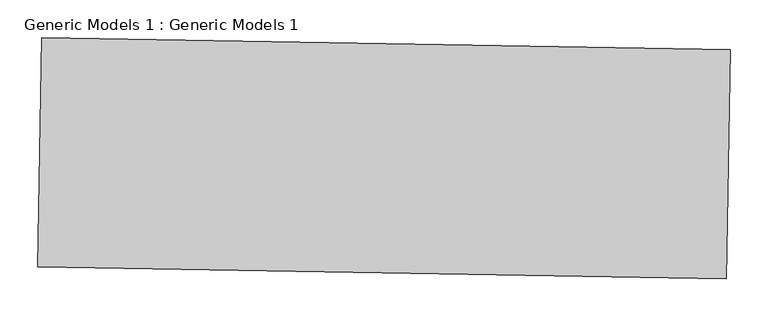
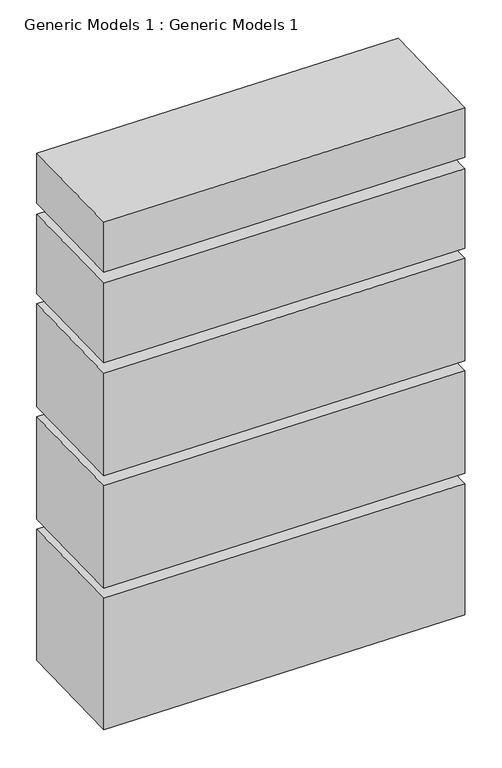
"""IFC4 building model written with IfcOpenShell, lengths in millimetres: proxy geometry, Generic Models 1 : Generic Models 1."""

from ifc_helpers import new_model, si_unit, frame, origin, place, context, project, spatial, polyline, outline, extrude, source, transform, mapped, element, save


def generic_models_1_generic_models_1_9302cbdc(model_context):
    return source(origin(), model_context, "Body", "SweptSolid", [
        extrude(outline(polyline([(-9021.9677264, -11490.7844781), (-9936.2284588, -11474.8259976), (-9930.9089653, -11170.0724201), (-9016.6482329, -11186.0309006), (-9021.9677264, -11490.7844781)])), frame((0.0, 0.0, 1263.5574996), z_axis=(0.0, 0.0, 1.0), x_axis=(1.0, 0.0, 0.0)), (0.0, 0.0, 1.0), 134.9289866),
        extrude(outline(polyline([(-9021.9677264, -11490.7844781), (-9936.2284588, -11474.8259976), (-9930.9089653, -11170.0724201), (-9016.6482329, -11186.0309006), (-9021.9677264, -11490.7844781)])), frame((0.0, 0.0, 26.8864862), z_axis=(0.0, 0.0, 1.0), x_axis=(1.0, 0.0, 0.0)), (0.0, 0.0, 1.0), 354.4191875),
        extrude(outline(polyline([(-9021.9677264, -11490.7844781), (-9936.2284588, -11474.8259976), (-9930.9089653, -11170.0724201), (-9016.6482329, -11186.0309006), (-9021.9677264, -11490.7844781)])), frame((0.0, 0.0, 1018.4973826), z_axis=(0.0, 0.0, 1.0), x_axis=(1.0, 0.0, 0.0)), (0.0, 0.0, 1.0), 214.5718039),
        extrude(outline(polyline([(-9021.9677264, -11490.7844781), (-9936.2284588, -11474.8259976), (-9930.9089653, -11170.0724201), (-9016.6482329, -11186.0309006), (-9021.9677264, -11490.7844781)])), frame((0.0, 0.0, 713.6973826), z_axis=(0.0, 0.0, 1.0), x_axis=(1.0, 0.0, 0.0)), (0.0, 0.0, 1.0), 277.2082911),
        extrude(outline(polyline([(-9021.9677264, -11490.7844781), (-9936.2284588, -11474.8259976), (-9930.9089653, -11170.0724201), (-9016.6482329, -11186.0309006), (-9021.9677264, -11490.7844781)])), frame((0.0, 0.0, 408.8973826), z_axis=(0.0, 0.0, 1.0), x_axis=(1.0, 0.0, 0.0)), (0.0, 0.0, 1.0), 277.2082911),
    ])


if __name__ == "__main__":
    model = new_model("IFC4")
    model_context = context("Model", 3, world=origin())
    ifc_project = project(units=[si_unit("LENGTHUNIT", "METRE", prefix="MILLI")], contexts=[model_context])
    site = spatial("IfcSite", under=ifc_project)
    building = spatial("IfcBuilding", under=site)
    placement = place(None, origin())
    generic_models_1_generic_models_1_shape = generic_models_1_generic_models_1_9302cbdc(model_context)
    element("IfcBuildingElementProxy", 1, Name="Generic Models 1 : Generic Models 1", ObjectType="Generic Models 1 : Generic Models 1", at=placement, inside=building, context=model_context, shape_type="MappedRepresentation", body=[
        mapped(generic_models_1_generic_models_1_shape, transform((0.0, 0.0, 0.0), x_axis=(1.0, 0.0, 0.0), y_axis=(0.0, 1.0, 0.0), z_axis=(0.0, 0.0, 1.0))),
    ])
    save(model, "model.ifc")

# Revit data of these elements
# Element 1 (IfcBuildingElementProxy, "Generic Models 1 : Generic Models 1")
#   Materials on its faces: "Parking Stripe"
# Materials
#   "Parking Stripe": class "Paint", colour RGB 250 250 91, transparency 0, Cost = 0
